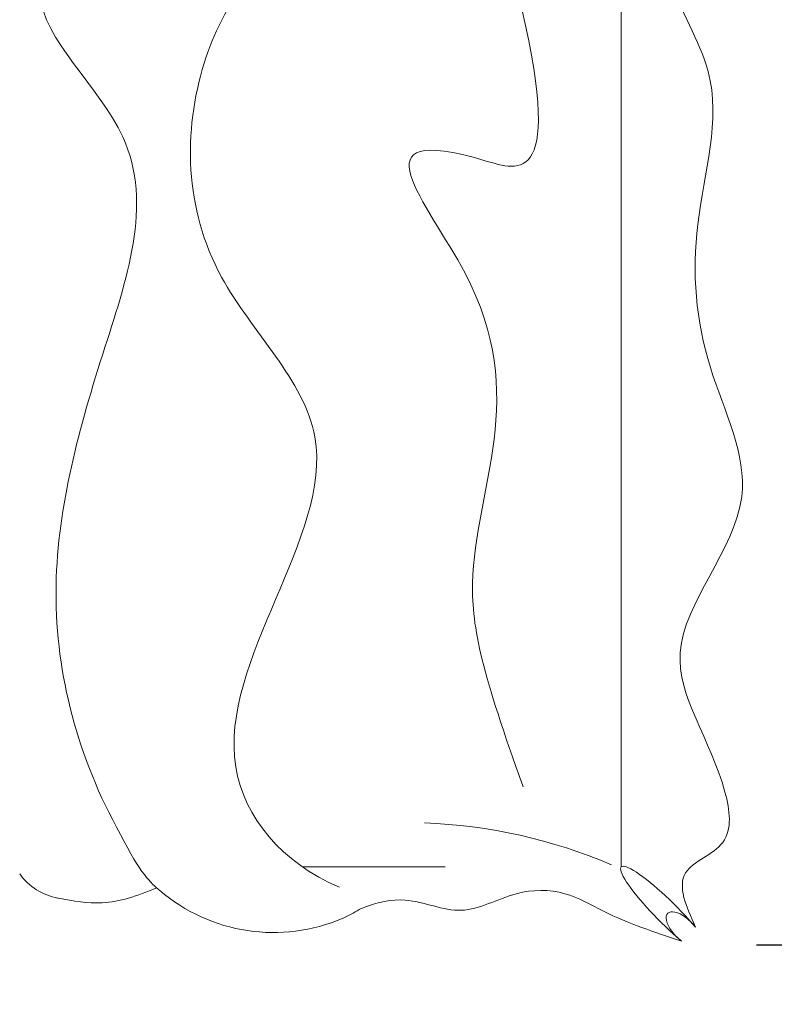
# Model space of a CAD drawing. Units: inches. Extents: x 2083 to 3317, y 1141 to 2115.
# Tile 97 of 256: x 2290 to 2339, y 1894 to 1958. Entities that reach past the tile are written whole.
import ezdxf

# ---------------------------------------------------------------- set-up
doc = ezdxf.new("R2010")
doc.units = ezdxf.units.IN
for name, color, linetype, lineweight in [('A-ANNO-DIMS', 2, 'Continuous', 18), ('A-FURN', 8, 'Continuous', 18), ('www.cadblocksfree.com', 7, 'Continuous', 9)]:
    doc.layers.add(name, color=color, linetype=linetype, lineweight=lineweight)
doc.layers.add('A-WALL-PATT', color=251, linetype='Continuous', lineweight=13, true_color=0x636466)
doc.styles.get("Standard").update_dxf_attribs({"font": 'arial.ttf'})
doc.dimstyles.new('ISO-25', dxfattribs={"dimtxt": 12, "dimasz": 12, "dimexe": 1.25, "dimexo": 0.625, "dimtad": 1, "dimlunit": 3, "dimtxsty": 'Standard', "dimcen": 2.5, "dimadec": 0, "dimazin": 0, "dimtfac": 1, "dimtmove": 0, "dimatfit": 3, "dimfxl": 1, "dimarcsym": 0})

# ---------------------------------------------------------------- blocks, each defined once
blk = doc.blocks.new('bed')
at = {"layer": 'www.cadblocksfree.com', "ltscale": 0.2}
for p, q in [((3363.387, 1412.3), (3363.387, 1402.937)), ((3363.387, 1391.414), (3426.379, 1391.414))]:
    blk.add_line(p, q, dxfattribs=at)
for centre, radius, start, end in [((3365.21, 1427.605), 3.937, 125.4209, 169.69818), ((3370.55, 1414.186), 11.465, 139.46484, 203.37116), ((3367.278, 1412.869), 7.939, 204.0179, 212.61896), ((3331.909, 1405.558), 34.378, 336.84952, 357.90025)]:
    blk.add_arc(centre, radius, start, end, dxfattribs=at)
at = {"layer": 'www.cadblocksfree.com', "ltscale": 0.2, "extrusion": (0, 0, -1)}
for centre, major_axis, ratio, start_param, end_param in [((3360.344, 1388.371), (3.043, 3.043), 0.168252, 4.250342, 8.316029), ((3359.289, 1387.316), (1.055, 1.055), 0.453532, 4.422107, 8.144264)]:
    blk.add_ellipse(centre, major_axis=major_axis, ratio=ratio, start_param=start_param, end_param=end_param, dxfattribs=at)
at = {"layer": 'www.cadblocksfree.com', "ltscale": 0.2}
for points, knots in [([(3365.512, 1424.213), (3370.519, 1427.004), (3381.149, 1429.825), (3396.214, 1425.866), (3410.541, 1420.654), (3420.273, 1432.695), (3425.882, 1426.771), (3428.534, 1423.97)], [0.099185, 0.099185, 0.099185, 0.099185, 0.523647, 0.927087, 1.289918, 1.564439, 1.810555, 1.810555, 1.810555, 1.810555]), ([(3361.336, 1428.309), (3361.334, 1428.297), (3361.16, 1427.338), (3360.778, 1425.173), (3361.469, 1423.14), (3362.014, 1421.845)], [0.3128349, 0.3128349, 0.3128349, 0.3128349, 0.313751, 0.386958, 0.4759027, 0.4759027, 0.4759027, 0.4759027]), ([(3362.057, 1409.866), (3363.638, 1413.65), (3372.978, 1421.337), (3389.682, 1406.045), (3402.396, 1419.984), (3416.037, 1420.167), (3423.233, 1415.231), (3427.827, 1408.899)], [0.029901, 0.029901, 0.029901, 0.029901, 0.276967, 0.797115, 1.093669, 1.464666, 1.788489, 1.788489, 1.788489, 1.788489]), ([(3368.632, 1397.839), (3375.978, 1400.489), (3385.349, 1402.757), (3397.531, 1395.273), (3413.593, 1410.377), (3407.806, 1395.019), (3420.759, 1398.2)], [0.029901, 0.029901, 0.029901, 0.029901, 0.276967, 0.797115, 1.093669, 1.16836, 1.16836, 1.16836, 1.16836]), ([(3358.529, 1387.473), (3359.098, 1389.205), (3359.955, 1391.816), (3361.924, 1395.149), (3361.896, 1398.555), (3359.883, 1401.841), (3361.557, 1405.208), (3361.034, 1407.507), (3360.643, 1408.467), (3360.591, 1408.59)], [0, 0, 0, 0, 0.138875, 0.2092702, 0.2901949, 0.3858479, 0.4804923, 0.5489252, 0.5590752, 0.5590752, 0.5590752, 0.5590752]), ([(3430.32, 1386.556), (3427.327, 1387.653), (3422.148, 1389.55), (3414.529, 1384.137), (3405.607, 1387.046), (3396.29, 1386.314), (3386.838, 1381.282), (3377.742, 1390.272), (3370.778, 1384.799), (3364.626, 1383.966), (3363.275, 1388.265), (3360.778, 1387.151), (3359.446, 1386.556)], [0, 0, 0, 0, 8.93042, 15.449194, 25.485629, 34.878505, 43.598887, 54.554403, 64.16647, 67.461673, 70.610457, 74.213583, 74.213583, 74.213583, 74.213583])]:
    blk.add_open_spline(points, degree=3, knots=knots, dxfattribs=at)
for points in [[(3361.235, 1424.042), (3361.236, 1424.042), (3361.237, 1424.043), (3361.239, 1424.043)], [(3361.837, 1421.637), (3362.352, 1422.25), (3362.867, 1422.863), (3365.512, 1424.213)]]:
    blk.add_open_spline(points, degree=3, dxfattribs=at)
blk = doc.blocks.new('*D21')
at = {"layer": 'A-ANNO-DIMS', "color": 0, "lineweight": -2, "transparency": 16777216}
for p, q in [((2351.181, 1970.691), (2351.181, 2057.153)), ((2337.845, 1970.691), (2352.431, 1970.691)), ((2351.181, 1909.744), (2351.181, 1958.691)), ((2337.845, 1897.744), (2352.431, 1897.744))]:
    blk.add_line(p, q, dxfattribs=at)
at = {"layer": 'A-ANNO-DIMS', "color": 0, "transparency": 16777216}
for points in [[(2349.181, 1958.691), (2353.181, 1958.691), (2351.181, 1970.691)], [(2349.181, 1909.744), (2353.181, 1909.744), (2351.181, 1897.744)]]:
    blk.add_solid(points, dxfattribs=at)
at = {"layer": 'Defpoints', "color": 0, "transparency": 16777216}
for p in [(2337.22, 1970.691), (2351.181, 1970.691), (2337.22, 1897.744)]:
    blk.add_point(p, dxfattribs=at)
at = {"layer": 'A-ANNO-DIMS', "color": 0, "transparency": 16777216, "insert": (2344.429, 2019.922), "char_height": 12, "attachment_point": 5, "rotation": 90}
blk.add_mtext('6\'-1" TYP.', dxfattribs=at)

msp = doc.modelspace()

# ---------------------------------------------------------------- hatches: boundary and pattern name
at = {"layer": 'A-WALL-PATT'}
h = msp.add_hatch(color=256, dxfattribs=at)
h.dxf.hatch_style = 1
h.paths.add_polyline_path([(3126.96, 2020.761), (2748.96, 2020.761), (2604.96, 2020.761), (2226.96, 2020.761), (2226.96, 1702.761), (2466.96, 1702.761), (2466.96, 1582.761), (2418.96, 1582.761), (2418.96, 1477.761), (2226.96, 1477.761), (2226.96, 1263.261), (2544.96, 1263.261), (2544.96, 1411.761), (2604.96, 1411.761), (2685.96, 1411.761), (2685.96, 1420.761), (2604.96, 1420.761), (2604.96, 1573.761), (2604.96, 1702.761), (2604.96, 2011.761), (2748.96, 2011.761), (2748.96, 1702.761), (2862.96, 1702.761), (2862.96, 1621.761), (2871.96, 1621.761), (2871.96, 1702.761), (2883.96, 1702.761), (2883.96, 1706.939, -0.026459), (2883.96, 1711.761), (2757.96, 1711.761), (2757.96, 1807.761), (2787.96, 1807.761), (2787.96, 1812.261), (2757.96, 1812.261), (2757.96, 2011.761), (2877.96, 2011.761), (2877.96, 1812.261), (2847.96, 1812.261), (2847.96, 1807.761), (2889.836, 1807.761), (2889.836, 1812.261), (2882.46, 1812.261), (2882.46, 2011.761), (3117.96, 2011.761), (3117.96, 1812.261), (2937.836, 1812.261), (2937.836, 1807.761), (2995.71, 1807.761), (2995.71, 1796.118), (3000.21, 1796.118), (3000.21, 1807.761), (3117.96, 1807.761), (3117.96, 1711.761), (3000.21, 1711.761), (3000.21, 1760.118), (2998.573, 1760.118, -0.020711), (2995.71, 1760.118), (2995.71, 1711.761), (2931.96, 1711.761), (2931.96, 1702.761), (3126.96, 1702.761)])
h.paths.add_polyline_path([(2471.46, 2011.761), (2471.46, 1810.011), (2462.717, 1810.011), (2462.717, 1805.511), (2505.96, 1805.511), (2505.96, 1810.011), (2475.96, 1810.011), (2475.96, 2011.761), (2595.96, 2011.761), (2595.96, 1810.011), (2565.96, 1810.011), (2565.96, 1805.511), (2595.96, 1805.511), (2595.96, 1711.761), (2235.96, 1711.761), (2235.96, 1805.511), (2353.71, 1805.511), (2353.71, 1796.054), (2358.21, 1796.054), (2358.21, 1805.511), (2414.717, 1805.511), (2414.717, 1810.011), (2235.96, 1810.011), (2235.96, 2011.761)], flags=16)
h.paths.add_polyline_path([(2270.205, 1994.61), (2270.205, 1970.61), (2246.205, 1970.61), (2246.205, 1994.61)], flags=0)
edge = h.paths.add_edge_path(flags=0)
edge.add_ellipse((2332.027, 1899.798), major_axis=(-3.043, 3.043), ratio=0.168252, start_angle=-161.33217, end_angle=-156.30711, ccw=False)
edge.add_ellipse((2333.082, 1898.744), major_axis=(-1.055, 1.055), ratio=0.453532, start_angle=-123.37102, end_angle=-94.15911)
edge = h.paths.add_edge_path(flags=0)
edge.add_ellipse((2332.027, 1968.876), major_axis=(3.043, 3.043), ratio=0.168252, start_angle=18.66783, end_angle=23.69289)
edge.add_spline(control_points=[(2332.926, 1970.691), (2332.227, 1970.336), (2330.894, 1969.659), (2328.413, 1970.932), (2327.204, 1967.749), (2324.71, 1969.956), (2322.533, 1967.012), (2320.013, 1971.296), (2317.68, 1968.158), (2316.041, 1967.102), (2315.427, 1966.81)], knot_values=[0, 0, 0, 0, 2.267059, 4.324559, 6.685584, 8.878641, 11.121502, 14.300359, 17.755284, 19.732645, 19.732645, 19.732645, 19.732645], degree=3, periodic=0)
edge.add_ellipse((2332.027, 1968.876), major_axis=(3.043, 3.043), ratio=0.168252, start_angle=18.66783, end_angle=23.69289, ccw=False)
edge.add_ellipse((2333.082, 1969.931), major_axis=(1.055, 1.055), ratio=0.453532, start_angle=56.62898, end_angle=85.84089, ccw=False)
edge = h.paths.add_edge_path(flags=0)
edge.add_spline(control_points=[(2296.428, 1967.988), (2293.628, 1965.336), (2287.704, 1959.727), (2299.744, 1949.996), (2294.533, 1935.669), (2290.573, 1920.604), (2293.394, 1909.974), (2296.185, 1904.967)], knot_values=[0.099185, 0.099185, 0.099185, 0.099185, 0.345301, 0.619822, 0.982653, 1.386093, 1.810555, 1.810555, 1.810555, 1.810555], degree=3, periodic=0)
edge.add_spline(control_points=[(2296.185, 1904.967), (2297.384, 1902.619), (2298.001, 1901.949), (2298.553, 1901.468)], knot_values=[0.006246, 0.006246, 0.006246, 0.006246, 0.055476, 0.055476, 0.055476, 0.055476], degree=3, periodic=0)
edge.add_spline(control_points=[(2298.553, 1901.468), (2297.259, 1900.923), (2295.225, 1900.232), (2293.06, 1900.614), (2292.101, 1900.788), (2292.09, 1900.791)], knot_values=[0.312835, 0.312835, 0.312835, 0.312835, 0.40178, 0.474987, 0.475903, 0.475903, 0.475903, 0.475903], degree=3, periodic=0)
edge.add_arc((2292.794, 1904.664), 3.937, 215.4209, 259.69818, ccw=False)
edge.add_spline(control_points=[(2289.585, 1902.382), (2289.477, 1902.535), (2289.368, 1902.688), (2289.261, 1902.841)], knot_values=[0.102872, 0.102872, 0.102872, 0.102872, 0.116896, 0.116896, 0.116896, 0.116896], degree=3, periodic=0)
edge.add_spline(control_points=[(2289.261, 1902.841), (2288.687, 1902.55), (2287.64, 1902.02), (2285.881, 1901.874), (2283.853, 1901.504), (2281.72, 1899.711), (2278.467, 1899.493), (2276.157, 1901.883), (2272.259, 1899.804), (2267.778, 1901.843), (2262.244, 1900.184), (2257.415, 1901.782), (2254.318, 1900.726), (2253.178, 1900.337)], knot_values=[0, 0, 0, 0, 1.907977, 3.477176, 5.261074, 7.972851, 11.680248, 13.717921, 16.939592, 22.789562, 27.502503, 33.595215, 37.145618, 37.145618, 37.145618, 37.145618], degree=3, periodic=0)
edge.add_line((2253.178, 1900.337), (2250.244, 1902.841))
edge.add_line((2250.244, 1902.841), (2250.244, 1965.833))
edge.add_line((2250.244, 1965.833), (2253.178, 1968.337))
edge.add_spline(control_points=[(2253.178, 1968.337), (2254.318, 1967.948), (2257.415, 1966.892), (2262.244, 1968.49), (2267.778, 1966.831), (2271.527, 1968.537), (2273.876, 1967.828), (2274.207, 1967.728)], knot_values=[0, 0, 0, 0, 0.09018, 0.244935, 0.364644, 0.513233, 0.537855, 0.537855, 0.537855, 0.537855], degree=3, periodic=0)
edge.add_arc((2274.353, 1963.793), 3.937, 72.05113, 92.12795, ccw=False)
edge.add_arc((2281.297, 1985.23), 18.596, 252.05113, 288.56572)
edge.add_arc((2292.317, 1956.029), 12.646, 71.02679, 113.77822, ccw=False)
edge = h.paths.add_edge_path(flags=0)
edge.add_spline(control_points=[(2274.899, 1951.856), (2275.066, 1951.617), (2275.233, 1951.377), (2275.398, 1951.136)], knot_values=[1.409916, 1.409916, 1.409916, 1.409916, 1.43159, 1.43159, 1.43159, 1.43159], degree=3, periodic=0)
edge.add_spline(control_points=[(2275.398, 1951.136), (2275.792, 1950.562), (2276.179, 1949.984), (2276.546, 1949.397)], knot_values=[1.358238, 1.358238, 1.358238, 1.358238, 1.409916, 1.409916, 1.409916, 1.409916], degree=3, periodic=0)
edge.add_line((2276.546, 1949.397), (2277.437, 1947.862))
edge.add_spline(control_points=[(2277.437, 1947.862), (2276.304, 1945.673), (2274.64, 1942.427), (2274.632, 1938.094), (2272.799, 1930.852), (2274.356, 1943.897), (2275.948, 1947.923), (2276.546, 1949.397)], knot_values=[0.005632, 0.005632, 0.005632, 0.005632, 0.186014, 0.266002, 0.357087, 0.59639, 0.739732, 0.739732, 0.739732, 0.739732], degree=3, periodic=0)
edge.add_spline(control_points=[(2276.546, 1949.397), (2276.179, 1949.984), (2275.792, 1950.562), (2275.398, 1951.136)], knot_values=[1.358238, 1.358238, 1.358238, 1.358238, 1.409916, 1.409916, 1.409916, 1.409916], degree=3, periodic=0)
edge.add_spline(control_points=[(2275.398, 1951.136), (2274.943, 1950.08), (2274.208, 1948.025), (2273.935, 1944.851), (2272.469, 1937.627), (2273.466, 1945.696), (2274.701, 1951.059), (2274.899, 1951.856)], knot_values=[0.104364, 0.104364, 0.104364, 0.104364, 0.189636, 0.269624, 0.36071, 0.600013, 0.644622, 0.644622, 0.644622, 0.644622], degree=3, periodic=0)
h.paths.add_polyline_path([(2269.168, 1963.128, -0.357527), (2268.171, 1960.976, -0.092561), (2268.171, 1939.436, -0.357527), (2269.168, 1937.285, -0.357527), (2267.016, 1938.282, -0.164785), (2254.686, 1938.282, -0.357527), (2252.534, 1937.285, -0.357527), (2253.531, 1939.436, -0.092561), (2253.531, 1960.976, -0.357527), (2252.534, 1963.128, -0.357527), (2254.686, 1962.131, -0.164785), (2267.016, 1962.131, -0.357527)], flags=0)
h.paths.add_polyline_path([(2248.874, 1967.802), (2248.874, 1957.028), (2249.458, 1957.028), (2249.458, 1911.647), (2248.874, 1911.647), (2248.874, 1900.873), (2246.512, 1900.873, 0.197327), (2244.15, 1902.457), (2244.15, 1966.218, 0.197327), (2246.512, 1967.802)], flags=0)
h.paths.add_polyline_path([(2269.168, 1931.389, -0.357527), (2268.171, 1929.238, -0.092561), (2268.171, 1907.698, -0.357527), (2269.168, 1905.547, -0.357527), (2267.016, 1906.544, -0.164785), (2254.686, 1906.544, -0.357527), (2252.534, 1905.547, -0.357527), (2253.531, 1907.698, -0.092561), (2253.531, 1929.238, -0.357527), (2252.534, 1931.389, -0.357527), (2254.686, 1930.392, -0.164785), (2267.016, 1930.392, -0.357527)], flags=0)
edge = h.paths.add_edge_path(flags=0)
edge.add_spline(control_points=[(2276.197, 1906.724), (2276.168, 1909.029), (2276.114, 1913.372), (2270.598, 1924.925), (2273.905, 1919.013), (2275.922, 1916.262), (2275.475, 1912.402), (2277.258, 1910.381), (2276.696, 1908.225), (2276.646, 1906.813), (2276.618, 1906.008)], knot_values=[0, 0, 0, 0, 8.61026, 16.221274, 18.843057, 23.804898, 27.440828, 29.356102, 31.203478, 33.650687, 33.650687, 33.650687, 33.650687], degree=3, periodic=0)
edge.add_spline(control_points=[(2276.618, 1906.008), (2276.623, 1905.624), (2276.498, 1904.629), (2275.442, 1903.855), (2274.937, 1903.08), (2274.859, 1902.841)], knot_values=[0.156488, 0.156488, 0.156488, 0.156488, 0.184398, 0.231376, 0.250598, 0.250598, 0.250598, 0.250598], degree=3, periodic=0)
edge.add_line((2274.859, 1902.841), (2276.506, 1902.841))
edge.add_spline(control_points=[(2276.506, 1902.841), (2276.788, 1903.085), (2277.665, 1904.125), (2278.25, 1904.341), (2277.654, 1908.527), (2278.156, 1906.228), (2278.1, 1905.286), (2278.847, 1904.069), (2277.857, 1903.415), (2277.874, 1902.991), (2277.904, 1902.841)], knot_values=[0.059574, 0.059574, 0.059574, 0.059574, 0.080753, 0.103741, 0.16972, 0.176036, 0.207137, 0.240474, 0.262341, 0.27366, 0.27366, 0.27366, 0.27366], degree=3, periodic=0)
edge.add_line((2277.904, 1902.841), (2280.03, 1902.841))
edge.add_spline(control_points=[(2280.03, 1902.841), (2279.888, 1903.088), (2279.499, 1903.982), (2280.152, 1905.939), (2278.104, 1909.658), (2279.762, 1907.185), (2280.328, 1904.875), (2280.485, 1903.49), (2281.463, 1903.249), (2281.758, 1902.936), (2281.834, 1902.841)], knot_values=[0.013856, 0.013856, 0.013856, 0.013856, 0.034874, 0.088867, 0.107879, 0.126738, 0.158714, 0.193757, 0.217487, 0.226722, 0.226722, 0.226722, 0.226722], degree=3, periodic=0)
edge.add_spline(control_points=[(2281.834, 1902.841), (2281.788, 1902.827), (2281.647, 1902.783), (2281.396, 1902.859), (2281.088, 1902.985), (2280.721, 1903.061), (2280.333, 1903.026), (2280.125, 1902.899), (2280.03, 1902.841)], knot_values=[0, 0, 0, 0, 0.14413, 0.435517, 0.749276, 1.153046, 1.548371, 1.878348, 1.878348, 1.878348, 1.878348], degree=3, periodic=0)
edge.add_line((2280.03, 1902.841), (2277.904, 1902.841))
edge.add_spline(control_points=[(2277.904, 1902.841), (2277.893, 1902.796), (2277.865, 1902.68), (2277.607, 1902.687), (2277.274, 1902.801), (2276.838, 1902.62), (2276.584, 1902.789), (2276.506, 1902.841)], knot_values=[0, 0, 0, 0, 0.127189, 0.326199, 0.628009, 1.24357, 1.515331, 1.515331, 1.515331, 1.515331], degree=3, periodic=0)
edge.add_line((2276.506, 1902.841), (2274.859, 1902.841))
edge.add_spline(control_points=[(2274.859, 1902.841), (2274.814, 1902.899), (2274.725, 1903.013), (2274.493, 1903.119), (2274.244, 1902.961), (2273.937, 1903.185), (2273.614, 1902.983), (2273.408, 1902.883), (2273.322, 1902.841)], knot_values=[0, 0, 0, 0, 0.21843, 0.436957, 0.687977, 0.990379, 1.398396, 1.69185, 1.69185, 1.69185, 1.69185], degree=3, periodic=0)
edge.add_spline(control_points=[(2273.322, 1902.841), (2273.617, 1903.446), (2274.274, 1904.538), (2276.027, 1904.574), (2276.207, 1906.584), (2276.197, 1906.724)], knot_values=[0.012227, 0.012227, 0.012227, 0.012227, 0.059472, 0.106218, 0.134458, 0.134458, 0.134458, 0.134458], degree=3, periodic=0)
h.paths.add_polyline_path([(2270.776, 1897.79), (2270.776, 1873.79), (2246.776, 1873.79), (2246.776, 1897.79)], flags=0)
h.paths.add_polyline_path([(2353.71, 1760.005), (2353.71, 1760.054), (2358.21, 1760.054, -0.033729)], flags=0)
h.paths.add_polyline_path([(2321.819, 1737.529), (2341.995, 1737.529, -0.414214), (2343.203, 1736.321), (2343.203, 1721.021, -0.414214), (2341.995, 1719.813), (2321.819, 1719.813, -0.414214), (2320.611, 1721.021), (2320.611, 1736.321, -0.414214)], flags=0)
h.paths.add_polyline_path([(2324.235, 1736.321), (2339.579, 1736.321, -0.414214), (2341.995, 1733.905), (2341.995, 1725.45, -0.414214), (2339.579, 1723.034), (2333.681, 1723.034), (2333.845, 1722.045, -0.870646), (2335.425, 1721.826, -0.767327), (2333.923, 1721.423), (2331.291, 1721.423, -0.767327), (2329.788, 1721.826, -0.870646), (2331.368, 1722.045), (2331.533, 1723.034), (2324.235, 1723.034, -0.414214), (2321.819, 1725.45), (2321.819, 1733.905, -0.414214)], flags=0)
h.paths.add_polyline_path([(2570.484, 1928.615), (2589.684, 1928.615), (2590.169, 1928.615), (2590.169, 1904.993), (2570.484, 1904.993)], flags=0)
h.paths.add_polyline_path([(2574.447, 1927.264, -1), (2572.829, 1927.264, -1)], flags=0)
h.paths.add_polyline_path([(2573.09, 1926.941), (2573.925, 1927.776), (2574.148, 1927.553), (2573.313, 1926.718)], flags=0)
h.paths.add_polyline_path([(2578.779, 1919.73, -1), (2571.592, 1919.73, -1)], flags=0)
h.paths.add_polyline_path([(2578.385, 1919.73, -1), (2571.985, 1919.73, -1)], flags=0)
h.paths.add_polyline_path([(2331.596, 1729.476, -1), (2333.618, 1729.476, -1)], flags=0)
h.paths.add_polyline_path([(2578.034, 1927.264, -1), (2576.416, 1927.264, -1)], flags=0)
h.paths.add_polyline_path([(2576.689, 1927.531), (2576.912, 1927.754), (2577.747, 1926.919), (2577.524, 1926.696)], flags=0)
h.paths.add_polyline_path([(2578.139, 1909.86, -1), (2572.232, 1909.86, -1)], flags=0)
h.paths.add_polyline_path([(2577.745, 1909.86, -1), (2572.625, 1909.86, -1)], flags=0)
h.paths.add_polyline_path([(2583.798, 1927.264, -1), (2582.179, 1927.264, -1)], flags=0)
h.paths.add_polyline_path([(2582.719, 1927.754), (2583.554, 1926.919), (2583.331, 1926.696), (2582.496, 1927.531)], flags=0)
h.paths.add_polyline_path([(2582.496, 1927.531), (2582.719, 1927.754), (2583.554, 1926.919), (2583.331, 1926.696)], flags=0)
h.paths.add_polyline_path([(2587.739, 1920.53, -1), (2581.832, 1920.53, -1)], flags=0)
h.paths.add_polyline_path([(2587.345, 1920.53, -1), (2582.225, 1920.53, -1)], flags=0)
h.paths.add_polyline_path([(2587.385, 1927.264, -1), (2585.766, 1927.264, -1)], flags=0)
h.paths.add_polyline_path([(2586.082, 1926.98), (2586.917, 1927.815), (2587.14, 1927.593), (2586.305, 1926.758)], flags=0)
h.paths.add_polyline_path([(2588.379, 1910.66, -1), (2581.192, 1910.66, -1)], flags=0)
h.paths.add_polyline_path([(2587.985, 1910.66, -1), (2581.585, 1910.66, -1)], flags=0)
h.paths.add_polyline_path([(2417.168, 1729.478), (2437.344, 1729.478, -0.414214), (2438.552, 1728.27), (2438.552, 1712.969, -0.414214), (2437.344, 1711.761), (2417.168, 1711.761, -0.414214), (2415.96, 1712.969), (2415.96, 1728.27, -0.414214)], flags=0)
h.paths.add_polyline_path([(2419.584, 1728.27), (2434.928, 1728.27, -0.414214), (2437.344, 1725.854), (2437.344, 1717.398, -0.414214), (2434.928, 1714.983), (2429.029, 1714.983), (2429.194, 1713.994, -0.870646), (2430.774, 1713.775, -0.767327), (2429.271, 1713.372), (2426.64, 1713.372, -0.767327), (2425.137, 1713.775, -0.870646), (2426.717, 1713.994), (2426.882, 1714.983), (2419.584, 1714.983, -0.414214), (2417.168, 1717.398), (2417.168, 1725.854, -0.414214)], flags=0)
h.paths.add_polyline_path([(2419.584, 1728.27), (2434.928, 1728.27, -0.414214), (2437.344, 1725.854), (2437.344, 1717.398, -0.414214), (2434.928, 1714.983), (2429.029, 1714.983), (2428.358, 1719.009), (2427.553, 1719.009), (2426.882, 1714.983), (2419.584, 1714.983, -0.414214), (2417.168, 1717.398), (2417.168, 1725.854, -0.414214)], flags=0)
h.paths.add_polyline_path([(2426.944, 1721.425, -1), (2428.967, 1721.425, -1)], flags=0)
h.paths.add_polyline_path([(2475.96, 1702.761), (2595.96, 1702.761), (2595.96, 1582.761), (2475.96, 1582.761)], flags=16)
h.paths.add_polyline_path([(2427.96, 1573.761), (2595.96, 1573.761), (2595.96, 1468.761), (2595.96, 1420.761), (2384.46, 1420.761), (2384.46, 1468.761), (2427.96, 1468.761)], flags=16)
h.paths.add_polyline_path([(2379.96, 1468.761), (2379.96, 1420.761), (2235.96, 1420.761), (2235.96, 1468.761)], flags=16)
h.paths.add_polyline_path([(2317.816, 1466.696), (2337.992, 1466.696, -0.414214), (2339.2, 1465.488), (2339.2, 1450.187, -0.414214), (2337.992, 1448.979), (2317.816, 1448.979, -0.414214), (2316.608, 1450.187), (2316.608, 1465.488, -0.414214)], flags=0)
h.paths.add_polyline_path([(2320.232, 1465.488), (2335.576, 1465.488, -0.414214), (2337.992, 1463.072), (2337.992, 1454.616, -0.414214), (2335.576, 1452.2), (2329.677, 1452.2), (2329.842, 1451.212, -0.870646), (2331.422, 1450.992, -0.767327), (2329.92, 1450.59), (2327.288, 1450.59, -0.767327), (2325.785, 1450.992, -0.870646), (2327.365, 1451.212), (2327.53, 1452.2), (2320.232, 1452.2, -0.414214), (2317.816, 1454.616), (2317.816, 1463.072, -0.414214)], flags=0)
h.paths.add_polyline_path([(2320.232, 1465.488), (2335.576, 1465.488, -0.414214), (2337.992, 1463.072), (2337.992, 1454.616, -0.414214), (2335.576, 1452.2), (2329.677, 1452.2), (2329.006, 1456.227), (2328.201, 1456.227), (2327.53, 1452.2), (2320.232, 1452.2, -0.414214), (2317.816, 1454.616), (2317.816, 1463.072, -0.414214)], flags=0)
h.paths.add_polyline_path([(2327.593, 1458.643, -1), (2329.615, 1458.643, -1)], flags=0)
h.paths.add_polyline_path([(2244.412, 1433.34), (2241.921, 1433.34, -0.414214), (2240.018, 1435.244), (2240.018, 1440.953, -0.414211), (2241.921, 1442.856), (2244.412, 1442.856, -1.976472)], flags=0)
h.paths.add_polyline_path([(2245.357, 1434.398, -0.414214), (2245.357, 1441.799, -2.144098)], flags=0)
h.paths.add_polyline_path([(2535.96, 1416.261), (2535.96, 1272.261), (2235.96, 1272.261), (2235.96, 1416.261)], flags=16)
h.paths.add_polyline_path([(2260.12, 1384.293), (2260.12, 1362.039), (2237.865, 1362.039), (2237.865, 1384.293)], flags=0)
edge = h.paths.add_edge_path(flags=0)
edge.add_line((2318.252, 1362.093), (2318.146, 1362.001))
edge.add_ellipse((2317.445, 1360.431), major_axis=(2.822, 2.822), ratio=0.168252, start_angle=18.66783, end_angle=20.94813, ccw=False)
edge.add_ellipse((2318.423, 1361.409), major_axis=(0.978, 0.978), ratio=0.453532, start_angle=56.62898, end_angle=70.2262, ccw=False)
edge = h.paths.add_edge_path(flags=0)
edge.add_line((2319.107, 1295.571), (2319.015, 1295.677))
edge.add_ellipse((2317.445, 1296.378), major_axis=(-2.822, 2.822), ratio=0.168252, start_angle=-161.33217, end_angle=-159.05187, ccw=False)
edge.add_ellipse((2318.423, 1295.4), major_axis=(-0.978, 0.978), ratio=0.453532, start_angle=-123.37102, end_angle=-109.7738)
edge = h.paths.add_edge_path(flags=0)
edge.add_spline(control_points=[(2284.21, 1301.17), (2284.581, 1300.445), (2284.891, 1299.892), (2285.16, 1299.461)], knot_values=[0.039066, 0.039066, 0.039066, 0.039066, 0.055476, 0.055476, 0.055476, 0.055476], degree=3, periodic=0)
edge.add_line((2285.16, 1299.461), (2284.21, 1301.17))
edge = h.paths.add_edge_path(flags=0)
edge.add_line((2280.412, 1297.298), (2283.37, 1297.036))
edge.add_line((2283.37, 1297.036), (2286.406, 1297.926))
edge.add_spline(control_points=[(2286.406, 1297.926), (2285.305, 1297.463), (2284.345, 1297.129), (2283.37, 1297.036)], knot_values=[0.394369, 0.394369, 0.394369, 0.394369, 0.475903, 0.475903, 0.475903, 0.475903], degree=3, periodic=0)
edge.add_spline(control_points=[(2283.37, 1297.036), (2283.281, 1297.028), (2282.316, 1296.957), (2281.313, 1297.134), (2280.423, 1297.296), (2280.412, 1297.298)], knot_values=[0.312835, 0.312835, 0.312835, 0.312835, 0.320246, 0.393453, 0.394369, 0.394369, 0.394369, 0.394369], degree=3, periodic=0)
edge = h.paths.add_edge_path(flags=0)
edge.add_line((2284.436, 1359.607), (2280.446, 1355.328))
edge.add_line((2280.446, 1355.328), (2279.58, 1351.018))
edge.add_line((2279.58, 1351.018), (2282.413, 1346.58))
edge.add_spline(control_points=[(2282.413, 1346.58), (2283.153, 1345.589), (2284.253, 1344.029), (2284.801, 1342.387), (2284.935, 1341.806)], knot_values=[1.240098, 1.240098, 1.240098, 1.240098, 1.332892, 1.382712, 1.382712, 1.382712, 1.382712], degree=3, periodic=0)
edge.add_spline(control_points=[(2284.935, 1341.806), (2285.319, 1340.141), (2285.233, 1338.409), (2284.91, 1336.654)], knot_values=[1.097484, 1.097484, 1.097484, 1.097484, 1.240098, 1.240098, 1.240098, 1.240098], degree=3, periodic=0)
edge.add_spline(control_points=[(2284.91, 1336.654), (2284.587, 1334.899), (2284.027, 1333.12), (2283.463, 1331.361)], knot_values=[0.95487, 0.95487, 0.95487, 0.95487, 1.097484, 1.097484, 1.097484, 1.097484], degree=3, periodic=0)
edge.add_line((2283.463, 1331.361), (2281.89, 1326.153))
edge.add_line((2281.89, 1326.153), (2280.756, 1321.056))
edge.add_line((2280.756, 1321.056), (2280.299, 1316.002))
edge.add_line((2280.299, 1316.002), (2280.716, 1310.95))
edge.add_line((2280.716, 1310.95), (2282.028, 1305.972))
edge.add_line((2282.028, 1305.972), (2284.21, 1301.17))
edge.add_spline(control_points=[(2284.21, 1301.17), (2283.341, 1302.73), (2282.612, 1304.336), (2282.028, 1305.972)], knot_values=[0.099185, 0.099185, 0.099185, 0.099185, 0.241799, 0.241799, 0.241799, 0.241799], degree=3, periodic=0)
edge.add_spline(control_points=[(2282.028, 1305.972), (2281.444, 1307.608), (2281.005, 1309.273), (2280.716, 1310.95)], knot_values=[0.241799, 0.241799, 0.241799, 0.241799, 0.384413, 0.384413, 0.384413, 0.384413], degree=3, periodic=0)
edge.add_spline(control_points=[(2280.716, 1310.95), (2280.433, 1312.588), (2280.289, 1314.277), (2280.299, 1315.962), (2280.299, 1316.002)], knot_values=[0.384413, 0.384413, 0.384413, 0.384413, 0.523647, 0.527028, 0.527028, 0.527028, 0.527028], degree=3, periodic=0)
edge.add_spline(control_points=[(2280.299, 1316.002), (2280.312, 1317.687), (2280.478, 1319.368), (2280.756, 1321.056)], knot_values=[0.527028, 0.527028, 0.527028, 0.527028, 0.669642, 0.669642, 0.669642, 0.669642], degree=3, periodic=0)
edge.add_spline(control_points=[(2280.756, 1321.056), (2281.035, 1322.744), (2281.426, 1324.44), (2281.89, 1326.153)], knot_values=[0.669642, 0.669642, 0.669642, 0.669642, 0.812256, 0.812256, 0.812256, 0.812256], degree=3, periodic=0)
edge.add_spline(control_points=[(2281.89, 1326.153), (2282.264, 1327.533), (2282.788, 1329.262), (2283.353, 1331.018), (2283.463, 1331.361)], knot_values=[0.812256, 0.812256, 0.812256, 0.812256, 0.927087, 0.95487, 0.95487, 0.95487, 0.95487], degree=3, periodic=0)
edge.add_line((2283.463, 1331.361), (2284.91, 1336.654))
edge.add_line((2284.91, 1336.654), (2284.935, 1341.806))
edge.add_line((2284.935, 1341.806), (2282.413, 1346.58))
edge.add_spline(control_points=[(2282.413, 1346.58), (2281.275, 1348.104), (2280.078, 1349.57), (2279.58, 1351.018)], knot_values=[1.382712, 1.382712, 1.382712, 1.382712, 1.525326, 1.525326, 1.525326, 1.525326], degree=3, periodic=0)
edge.add_spline(control_points=[(2279.58, 1351.018), (2279.443, 1351.415), (2279.136, 1352.857), (2279.735, 1354.29), (2280.446, 1355.328)], knot_values=[1.525326, 1.525326, 1.525326, 1.525326, 1.564439, 1.667941, 1.667941, 1.667941, 1.667941], degree=3, periodic=0)
edge.add_spline(control_points=[(2280.446, 1355.328), (2281.426, 1356.758), (2282.931, 1358.183), (2284.436, 1359.607)], knot_values=[1.667941, 1.667941, 1.667941, 1.667941, 1.810555, 1.810555, 1.810555, 1.810555], degree=3, periodic=0)
edge.add_arc((2280.623, 1348.518), 11.726, 71.02679, 113.77822)
edge.add_arc((2270.405, 1375.595), 17.244, 252.05113, 288.56572, ccw=False)
edge.add_arc((2263.966, 1355.718), 3.651, 72.05113, 92.12795)
edge.add_arc((2263.966, 1355.718), 3.651, 92.12795, 177.98513)
edge.add_spline(control_points=[(2260.318, 1355.846), (2260.26, 1354.221), (2260.551, 1350.187), (2262.999, 1346.766), (2264.473, 1344.649)], knot_values=[1.43159, 1.43159, 1.43159, 1.43159, 1.564144, 1.770695, 1.770695, 1.770695, 1.770695], degree=3, periodic=0)
edge.add_line((2264.473, 1344.649), (2264.936, 1343.983))
edge.add_spline(control_points=[(2263.801, 1340.248), (2263.843, 1340.514), (2264.067, 1341.756), (2264.513, 1343.002), (2264.935, 1343.981)], knot_values=[0.53657, 0.53657, 0.53657, 0.53657, 0.559349, 0.644622, 0.644622, 0.644622, 0.644622], degree=3, periodic=0)
edge.add_spline(control_points=[(2264.935, 1343.981), (2265.118, 1343.715), (2265.299, 1343.448), (2265.477, 1343.179)], knot_values=[1.384077, 1.384077, 1.384077, 1.384077, 1.409916, 1.409916, 1.409916, 1.409916], degree=3, periodic=0)
edge.add_spline(control_points=[(2265.477, 1343.179), (2265.655, 1342.911), (2265.829, 1342.641), (2265.999, 1342.369)], knot_values=[1.358238, 1.358238, 1.358238, 1.358238, 1.384077, 1.384077, 1.384077, 1.384077], degree=3, periodic=0)
edge.add_line((2265.999, 1342.369), (2266.826, 1340.946))
edge.add_spline(control_points=[(2266.826, 1340.946), (2268.894, 1337.09), (2271.398, 1325.843), (2270.516, 1310.569), (2275.919, 1301.861), (2277.79, 1299.199)], knot_values=[0.116896, 0.116896, 0.116896, 0.116896, 0.472987, 1.050969, 1.313793, 1.313793, 1.313793, 1.313793], degree=3, periodic=0)
edge.add_spline(control_points=[(2277.79, 1299.199), (2277.839, 1299.128), (2277.889, 1299.057), (2277.94, 1298.987)], knot_values=[0.109884, 0.109884, 0.109884, 0.109884, 0.116896, 0.116896, 0.116896, 0.116896], degree=3, periodic=0)
edge.add_line((2277.94, 1298.987), (2277.789, 1299.199))
edge.add_spline(control_points=[(2277.789, 1299.199), (2277.257, 1298.929), (2276.286, 1298.438), (2275.039, 1298.334), (2274.383, 1298.239), (2274.215, 1298.209)], knot_values=[33.12187, 33.12187, 33.12187, 33.12187, 35.029056, 36.598255, 37.144827, 37.144827, 37.144827, 37.144827], degree=3, periodic=0)
edge.add_line((2274.215, 1298.209), (2273.073, 1297.893))
edge.add_spline(control_points=[(2273.073, 1297.893), (2272.323, 1297.58), (2271.039, 1296.511), (2269.248, 1296.226), (2268.423, 1296.375)], knot_values=[26.532584, 26.532584, 26.532584, 26.532584, 29.198919, 31.839101, 31.839101, 31.839101, 31.839101], degree=3, periodic=0)
edge.add_line((2268.423, 1296.375), (2263.879, 1297.458))
edge.add_spline(control_points=[(2263.879, 1297.458), (2263.556, 1297.359), (2261.86, 1296.839), (2260.239, 1297.282), (2258.933, 1297.516)], knot_values=[15.919551, 15.919551, 15.919551, 15.919551, 16.939592, 21.226067, 21.226067, 21.226067, 21.226067], degree=3, periodic=0)
edge.add_line((2258.933, 1297.516), (2254.055, 1297.329))
edge.add_spline(control_points=[(2254.055, 1297.329), (2253.756, 1297.296), (2252.114, 1297.165), (2250.462, 1297.544), (2249.13, 1297.668)], knot_values=[5.306517, 5.306517, 5.306517, 5.306517, 6.276435, 10.613034, 10.613034, 10.613034, 10.613034], degree=3, periodic=0)
edge.add_line((2249.13, 1297.668), (2244.332, 1296.878))
edge.add_line((2244.332, 1296.878), (2241.611, 1299.199))
edge.add_line((2241.611, 1299.199), (2241.611, 1357.609))
edge.add_line((2241.611, 1357.609), (2244.332, 1359.931))
edge.add_line((2244.332, 1359.931), (2252.729, 1359.543))
edge.add_spline(control_points=[(2252.729, 1359.543), (2252.871, 1359.546), (2253.306, 1359.548), (2253.74, 1359.514), (2254.032, 1359.482)], knot_values=[0.233291, 0.233291, 0.233291, 0.233291, 0.244935, 0.268927, 0.268927, 0.268927, 0.268927], degree=3, periodic=0)
edge.add_line((2254.032, 1359.482), (2259.587, 1359.416))
edge.add_spline(control_points=[(2259.587, 1359.416), (2260.677, 1359.629), (2262.073, 1359.897), (2263.524, 1359.459), (2263.83, 1359.366)], knot_values=[0.422516, 0.422516, 0.422516, 0.422516, 0.513233, 0.537855, 0.537855, 0.537855, 0.537855], degree=3, periodic=0)
edge.add_arc((2263.966, 1355.718), 3.651, 72.05113, 92.12795, ccw=False)
edge.add_arc((2270.405, 1375.595), 17.244, 252.05113, 288.56572)
edge.add_arc((2280.623, 1348.518), 11.726, 71.02679, 113.77822, ccw=False)
h.paths.add_polyline_path([(2240.341, 1359.435), (2240.341, 1349.444), (2240.882, 1349.444), (2240.882, 1307.365), (2240.341, 1307.365), (2240.341, 1297.374), (2238.15, 1297.374, 0.197327), (2235.96, 1298.843), (2235.96, 1357.966, 0.197327), (2238.15, 1359.435)], flags=0)
h.paths.add_polyline_path([(2259.158, 1355.101, -0.357527), (2258.233, 1353.106, -0.092561), (2258.233, 1333.133, -0.357527), (2259.158, 1331.138, -0.357527), (2257.163, 1332.062, -0.164785), (2245.729, 1332.062, -0.357527), (2243.735, 1331.138, -0.357527), (2244.659, 1333.133, -0.092561), (2244.659, 1353.106, -0.357527), (2243.735, 1355.101, -0.357527), (2245.729, 1354.176, -0.164785), (2257.163, 1354.176, -0.357527)], flags=0)
edge = h.paths.add_edge_path(flags=0)
edge.add_line((2265.999, 1342.369), (2266.826, 1340.946))
edge.add_line((2266.826, 1340.946), (2265.308, 1337.814))
edge.add_line((2265.308, 1337.814), (2264.358, 1334.653))
edge.add_line((2264.358, 1334.653), (2264.262, 1333.8))
edge.add_spline(control_points=[(2264.262, 1333.8), (2264.208, 1333.187), (2264.162, 1332.366), (2264.007, 1331.414), (2263.969, 1331.202)], knot_values=[0.464444, 0.464444, 0.464444, 0.464444, 0.516691, 0.531608, 0.531608, 0.531608, 0.531608], degree=3, periodic=0)
edge.add_spline(control_points=[(2263.969, 1331.202), (2263.775, 1330.119), (2263.424, 1328.791), (2263.257, 1328.531), (2263.234, 1328.515)], knot_values=[0.372682, 0.372682, 0.372682, 0.372682, 0.44885, 0.464444, 0.464444, 0.464444, 0.464444], degree=3, periodic=0)
edge.add_spline(control_points=[(2263.234, 1328.515), (2263.096, 1328.42), (2263.131, 1329.301), (2263.275, 1330.616)], knot_values=[0.280919, 0.280919, 0.280919, 0.280919, 0.372682, 0.372682, 0.372682, 0.372682], degree=3, periodic=0)
edge.add_spline(control_points=[(2263.275, 1330.616), (2263.419, 1331.93), (2263.672, 1333.677), (2263.97, 1335.315)], knot_values=[0.189157, 0.189157, 0.189157, 0.189157, 0.280919, 0.280919, 0.280919, 0.280919], degree=3, periodic=0)
edge.add_spline(control_points=[(2263.97, 1335.315), (2264.1, 1336.032), (2264.419, 1337.622), (2264.755, 1338.864), (2264.947, 1339.491)], knot_values=[0.097394, 0.097394, 0.097394, 0.097394, 0.137578, 0.189157, 0.189157, 0.189157, 0.189157], degree=3, periodic=0)
edge.add_spline(control_points=[(2264.947, 1339.491), (2265.29, 1340.606), (2265.644, 1341.494), (2265.999, 1342.369)], knot_values=[0.005632, 0.005632, 0.005632, 0.005632, 0.097394, 0.097394, 0.097394, 0.097394], degree=3, periodic=0)
h.paths.add_polyline_path([(2259.158, 1325.671, -0.357527), (2258.233, 1323.676, -0.092561), (2258.233, 1303.703, -0.357527), (2259.158, 1301.708, -0.357527), (2257.163, 1302.633, -0.164785), (2245.729, 1302.633, -0.357527), (2243.735, 1301.708, -0.357527), (2244.659, 1303.703, -0.092561), (2244.659, 1323.676, -0.357527), (2243.735, 1325.671, -0.357527), (2245.729, 1324.747, -0.164785), (2257.163, 1324.747, -0.357527)], flags=0)
edge = h.paths.add_edge_path(flags=0)
edge.add_spline(control_points=[(2261.709, 1317.311), (2261.679, 1317.418), (2261.762, 1317.389), (2262.491, 1316.09), (2262.962, 1315.301)], knot_values=[14.955861, 14.955861, 14.955861, 14.955861, 16.221274, 18.694826, 18.694826, 18.694826, 18.694826], degree=3, periodic=0)
edge.add_spline(control_points=[(2262.962, 1315.301), (2262.99, 1315.254), (2263.702, 1314.067), (2264.349, 1313.127), (2264.73, 1312.164)], knot_values=[18.694826, 18.694826, 18.694826, 18.694826, 18.843057, 22.433791, 22.433791, 22.433791, 22.433791], degree=3, periodic=0)
edge.add_spline(control_points=[(2264.73, 1312.164), (2264.876, 1311.796), (2265.177, 1310.77), (2265.143, 1309.559), (2265.248, 1308.824)], knot_values=[22.433791, 22.433791, 22.433791, 22.433791, 23.804898, 26.172756, 26.172756, 26.172756, 26.172756], degree=3, periodic=0)
edge.add_line((2265.248, 1308.824), (2265.851, 1307.172))
edge.add_spline(control_points=[(2265.851, 1307.172), (2266.065, 1306.822), (2266.384, 1306.332), (2266.424, 1305.781), (2266.42, 1305.611)], knot_values=[28.062562, 28.062562, 28.062562, 28.062562, 29.356102, 29.911721, 29.911721, 29.911721, 29.911721], degree=3, periodic=0)
edge.add_spline(control_points=[(2266.42, 1305.611), (2266.416, 1305.433), (2266.394, 1305.25), (2266.365, 1305.066)], knot_values=[29.911721, 29.911721, 29.911721, 29.911721, 30.497837, 30.497837, 30.497837, 30.497837], degree=3, periodic=0)
edge.add_line((2266.365, 1305.066), (2266.066, 1302.136))
edge.add_spline(control_points=[(2266.066, 1302.136), (2266.071, 1301.78), (2265.998, 1301.2), (2265.663, 1300.759), (2265.509, 1300.586)], knot_values=[0.156488, 0.156488, 0.156488, 0.156488, 0.184398, 0.203543, 0.203543, 0.203543, 0.203543], degree=3, periodic=0)
edge.add_line((2265.509, 1300.586), (2264.435, 1299.199))
edge.add_line((2264.435, 1299.199), (2265.962, 1299.199))
edge.add_line((2265.962, 1299.199), (2267.336, 1301.175))
edge.add_line((2267.336, 1301.175), (2267.312, 1301.986))
edge.add_spline(control_points=[(2267.312, 1301.986), (2267.261, 1302.862), (2267.16, 1303.737), (2267.271, 1303.326)], knot_values=[0.126229, 0.126229, 0.126229, 0.126229, 0.166617, 0.166617, 0.166617, 0.166617], degree=3, periodic=0)
edge.add_spline(control_points=[(2267.271, 1303.326), (2267.28, 1303.294), (2267.31, 1303.175), (2267.373, 1302.884), (2267.406, 1302.683), (2267.418, 1302.601)], knot_values=[0.166617, 0.166617, 0.166617, 0.166617, 0.16972, 0.176036, 0.180765, 0.180765, 0.180765, 0.180765], degree=3, periodic=0)
edge.add_spline(control_points=[(2267.744, 1300.988), (2267.688, 1301.151), (2267.481, 1301.657), (2267.484, 1302.145), (2267.418, 1302.601)], knot_values=[0.180765, 0.180765, 0.180765, 0.180765, 0.193767, 0.220139, 0.220139, 0.220139, 0.220139], degree=3, periodic=0)
edge.add_line((2267.418, 1302.601), (2267.744, 1300.988))
edge.add_spline(control_points=[(2267.744, 1300.988), (2267.832, 1300.732), (2267.932, 1300.31), (2267.555, 1299.975), (2267.429, 1299.829)], knot_values=[0.220139, 0.220139, 0.220139, 0.220139, 0.240474, 0.25489, 0.25489, 0.25489, 0.25489], degree=3, periodic=0)
edge.add_line((2267.429, 1299.829), (2267.258, 1299.199))
edge.add_line((2267.258, 1299.199), (2269.23, 1299.199))
edge.add_spline(control_points=[(2269.23, 1299.199), (2269.099, 1299.429), (2268.843, 1300.016), (2269.012, 1300.916), (2268.947, 1301.661)], knot_values=[0.013856, 0.013856, 0.013856, 0.013856, 0.034874, 0.067073, 0.067073, 0.067073, 0.067073], degree=3, periodic=0)
edge.add_line((2268.947, 1301.661), (2268.432, 1303.603))
edge.add_spline(control_points=[(2268.432, 1303.603), (2268.176, 1304.192), (2267.596, 1305.251), (2268.041, 1304.623), (2268.251, 1304.282)], knot_values=[0.090155, 0.090155, 0.090155, 0.090155, 0.107879, 0.120289, 0.120289, 0.120289, 0.120289], degree=3, periodic=0)
edge.add_spline(control_points=[(2268.251, 1304.282), (2268.361, 1304.105), (2269.058, 1302.918), (2269.383, 1301.59), (2269.521, 1300.776), (2269.575, 1300.556)], knot_values=[0.120289, 0.120289, 0.120289, 0.120289, 0.126738, 0.158714, 0.173506, 0.173506, 0.173506, 0.173506], degree=3, periodic=0)
edge.add_line((2269.575, 1300.556), (2270.686, 1299.421))
edge.add_spline(control_points=[(2270.686, 1299.421), (2270.767, 1299.357), (2270.838, 1299.281), (2270.903, 1299.199)], knot_values=[0.21816, 0.21816, 0.21816, 0.21816, 0.226722, 0.226722, 0.226722, 0.226722], degree=3, periodic=0)
edge.add_line((2270.937, 1299.193), (2270.903, 1299.199))
edge.add_spline(control_points=[(2270.903, 1299.199), (2270.86, 1299.186), (2270.73, 1299.146), (2270.496, 1299.216), (2270.272, 1299.308), (2270.121, 1299.348), (2270.063, 1299.36)], knot_values=[0.939174, 0.939174, 0.939174, 0.939174, 1.083304, 1.374691, 1.68845, 1.878348, 1.878348, 1.878348, 1.878348], degree=3, periodic=0)
edge.add_line((2270.063, 1299.36), (2269.23, 1299.199))
edge.add_line((2269.23, 1299.199), (2267.258, 1299.199))
edge.add_spline(control_points=[(2267.258, 1299.199), (2267.248, 1299.157), (2267.223, 1299.05), (2266.984, 1299.057), (2266.809, 1299.116), (2266.677, 1299.109), (2266.637, 1299.105)], knot_values=[0.757665, 0.757665, 0.757665, 0.757665, 0.884854, 1.083864, 1.385675, 1.515331, 1.515331, 1.515331, 1.515331], degree=3, periodic=0)
edge.add_spline(control_points=[(2266.637, 1299.105), (2266.485, 1299.089), (2266.236, 1299.017), (2266.035, 1299.151), (2265.962, 1299.199)], knot_values=[0, 0, 0, 0, 0.485905, 0.757665, 0.757665, 0.757665, 0.757665], degree=3, periodic=0)
edge.add_line((2265.962, 1299.199), (2264.435, 1299.199))
edge.add_line((2264.435, 1299.199), (2263.858, 1299.367))
edge.add_spline(control_points=[(2263.858, 1299.367), (2263.819, 1299.371), (2263.78, 1299.386), (2263.74, 1299.402)], knot_values=[0.845925, 0.845925, 0.845925, 0.845925, 0.978627, 0.978627, 0.978627, 0.978627], degree=3, periodic=0)
edge.add_line((2263.722, 1299.396), (2263.01, 1299.199))
edge.add_spline(control_points=[(2263.01, 1299.199), (2263.246, 1299.683), (2263.506, 1300.128), (2263.873, 1300.408)], knot_values=[0.012227, 0.012227, 0.012227, 0.012227, 0.052971, 0.052971, 0.052971, 0.052971], degree=3, periodic=0)
edge.add_spline(control_points=[(2263.873, 1300.408), (2263.932, 1300.453), (2264.084, 1300.553), (2264.255, 1300.624), (2264.36, 1300.665)], knot_values=[0.052971, 0.052971, 0.052971, 0.052971, 0.059472, 0.069086, 0.069086, 0.069086, 0.069086], degree=3, periodic=0)
edge.add_line((2264.36, 1300.665), (2265.142, 1301.078))
edge.add_line((2265.142, 1301.078), (2265.676, 1302.8))
edge.add_line((2265.676, 1302.8), (2265.541, 1305.704))
edge.add_line((2265.541, 1305.704), (2264.803, 1309.328))
edge.add_line((2264.803, 1309.328), (2263.041, 1314.092))
edge.add_spline(control_points=[(2263.041, 1314.092), (2262.384, 1315.671), (2261.796, 1316.998), (2261.709, 1317.311)], knot_values=[11.216896, 11.216896, 11.216896, 11.216896, 14.955861, 14.955861, 14.955861, 14.955861], degree=3, periodic=0)
h.paths.add_polyline_path([(2871.96, 1416.261), (2895.91, 1416.261), (2895.91, 1420.761), (2871.96, 1420.761), (2871.96, 1501.761), (2862.96, 1501.761), (2862.96, 1420.761), (2805.96, 1420.761), (2805.96, 1411.761), (2862.96, 1411.761), (2862.96, 1263.261), (3126.96, 1263.261), (3126.96, 1411.761), (3126.96, 1486.761), (2943.96, 1486.761), (2943.96, 1477.761), (2967.86, 1477.761), (2967.86, 1420.761), (2943.91, 1420.761), (2943.91, 1416.261), (3117.96, 1416.261), (3117.96, 1420.761), (2972.36, 1420.761), (2972.36, 1477.761), (3117.96, 1477.761), (3117.96, 1420.761), (3117.96, 1272.261), (2871.96, 1272.261)], flags=0)
h.paths.add_polyline_path([(2457.126, 1485.943), (2527.603, 1485.943), (2527.603, 1537.636), (2457.126, 1537.636)], flags=8)
h.paths.add_polyline_path([(2481.005, 1609.982), (2590.766, 1609.982), (2590.766, 1682.003), (2481.005, 1682.003)], flags=8)
h.paths.add_polyline_path([(2483.085, 1729.127), (2553.562, 1729.127), (2553.562, 1780.82), (2483.085, 1780.82)], flags=8)

# ---------------------------------------------------------------- block references
at = {"layer": 'A-FURN', "rotation": 90}
msp.add_blockref('bed', (3720.398, -1460.546), dxfattribs=at)

# ---------------------------------------------------------------- dimensions: what is measured, and where the dimension line sits
at = {"layer": 'A-ANNO-DIMS'}
dim = msp.add_linear_dim(base=(2351.181, 1970.691), p1=(2337.22, 1897.744), p2=(2337.22, 1970.691), angle=90, text='<> TYP.', dimstyle='ISO-25', override={"dimdec": 1, "dimlfac": 1, "dimrnd": 0, "dimzin": 1, "dimdsep": 46, "dimlunit": 4, "dimfrac": 2}, dxfattribs=at)
dim.commit()
dim.dimension.update_dxf_attribs({"geometry": '*D21', "text_midpoint": (2344.429, 2019.922)})

doc.saveas('drawing.dxf')
